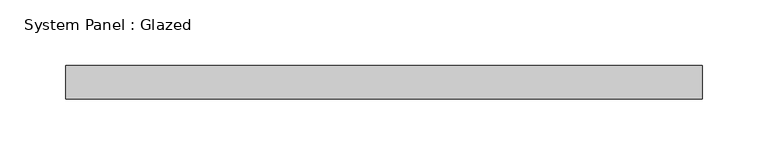
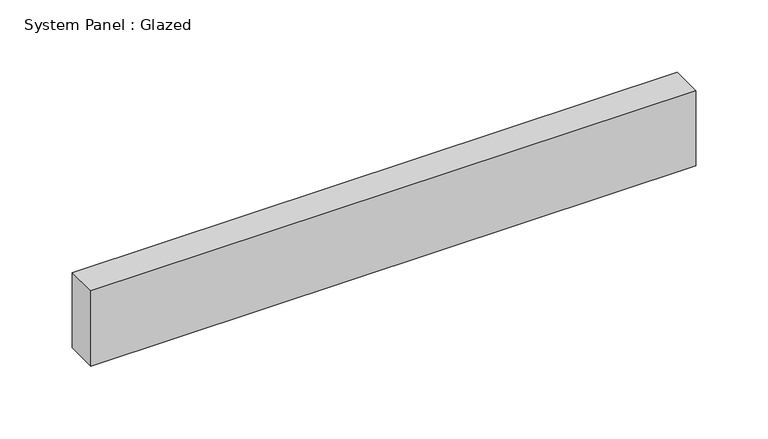
"""IFC4 building model written with IfcOpenShell, lengths in millimetres: plate geometry, System Panel : Glazed."""

from ifc_helpers import new_model, si_unit, origin, origin_with_axes, place, context, project, spatial, polyline, outline, extrude, source, transform, mapped, element, save


def system_panel_glazed_ee894bee(model_context):
    return source(origin(), model_context, "Body", "SweptSolid", [
        extrude(outline(polyline([(241.3, 19.05), (-241.3, 19.05), (-241.3, 44.45), (241.3, 44.45), (241.3, 19.05)])), origin_with_axes(), (0.0, 0.0, 1.0), 63.5),
    ])


if __name__ == "__main__":
    model = new_model("IFC4")
    model_context = context("Model", 3, world=origin())
    ifc_project = project(units=[si_unit("LENGTHUNIT", "METRE", prefix="MILLI")], contexts=[model_context])
    site = spatial("IfcSite", under=ifc_project)
    building = spatial("IfcBuilding", under=site)
    placement = place(None, origin())
    system_panel_glazed_shape = system_panel_glazed_ee894bee(model_context)
    element("IfcPlate", 1, ObjectType="System Panel : Glazed", at=placement, inside=building, context=model_context, shape_type="MappedRepresentation", body=[
        mapped(system_panel_glazed_shape, transform((0.0, 0.0, 0.0), x_axis=(1.0, 0.0, 0.0), y_axis=(0.0, 1.0, 0.0), z_axis=(0.0, 0.0, 1.0))),
    ])
    save(model, "model.ifc")

# Revit data of these elements
# Type "System Panel : Glazed"
#   Construction Type Id = "GSP4R"
#   Analytic Construction = "1/8 in Pilkington single glazing"
#   Visual Light Transmittance = 0.9
#   Solar Heat Gain Coefficient = 0.86
#   Heat Transfer Coefficient (U) = 1.18115 BTU/(h·ft²·°F)
#   Define Thermal Properties by = 1
# Element 1 (IfcPlate, "System Panel : Glazed")
#   Materials on its faces: "Glass"
# Materials
#   "Glass": class "Glass", colour RGB 0 128 192, transparency 0.75, Description = "Soda Lime Glass", Cost = 0
